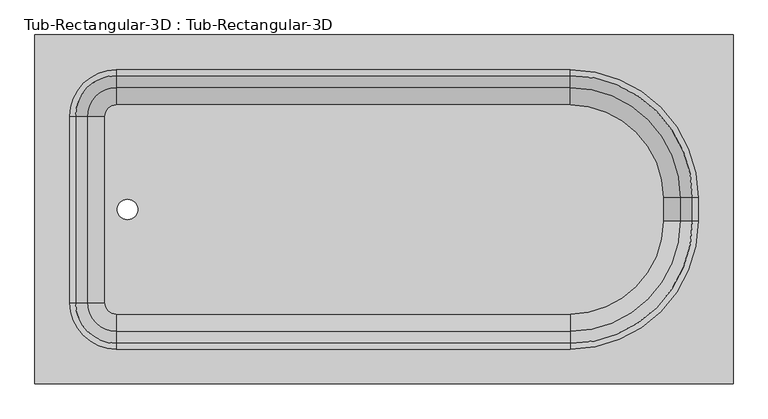
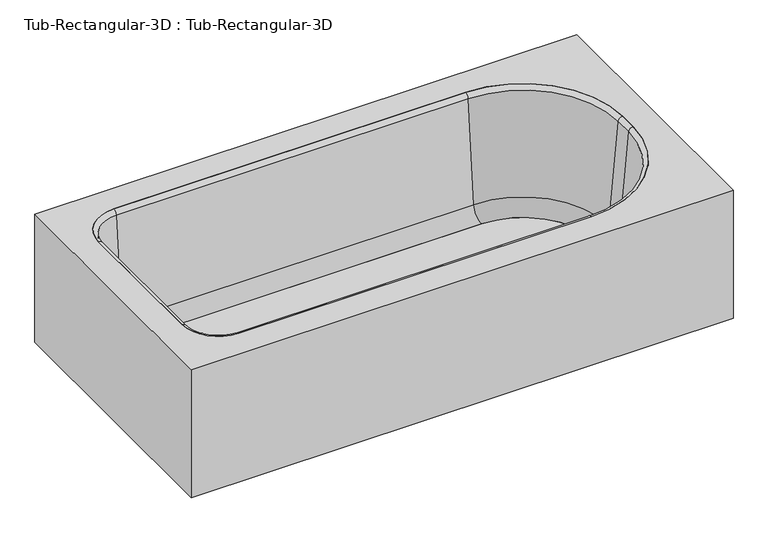
"""IFC4 building model written with IfcOpenShell, lengths in millimetres: flow terminal geometry, Tub-Rectangular-3D : Tub-Rectangular-3D."""

from ifc_helpers import new_model, si_unit, point, frame, frame_2d, origin, place, context, project, spatial, polyline, circle_curve, ellipse_curve, trimmed, segment, composite_curve, outline, extrude, source, transform, mapped, element, save
from ifc_brep_helpers import plane_surface, cylinder_surface, revolved_surface, advanced_brep


def tub_rectangular_3d_tub_rectangular_3d_36e24cee(model_context):
    return source(origin(), model_context, "Body", "SolidModel", [
        advanced_brep(
        [(413.3970313, 838.2, 381.0), (-1110.6029687, 838.2, 381.0), (-1110.6029687, 76.2, 381.0), (413.3970313, 76.2, 381.0), (-932.8029687, 762.0, 381.0), (57.7970313, 762.0, 381.0), (337.1970313, 482.6, 381.0), (337.1970313, 431.8, 381.0), (57.7970313, 152.4, 381.0), (-932.8029687, 152.4, 381.0), (-1034.4029687, 254.0, 381.0), (-1034.4029687, 660.4, 381.0), (394.3470313, 819.15, 361.95), (394.3470313, 95.25, 361.95), (-1091.5529687, 95.25, 361.95), (-1091.5529687, 819.15, 361.95), (-932.8029687, 762.0, 361.95), (-1034.4029687, 660.4, 361.95), (-1034.4029687, 254.0, 361.95), (-932.8029687, 152.4, 361.95), (57.7970313, 152.4, 361.95), (337.1970313, 431.8, 361.95), (337.1970313, 482.6, 361.95), (57.7970313, 762.0, 361.95), (413.3970313, 838.2, 0.0), (-1110.6029687, 838.2, 0.0), (-1110.6029687, 76.2, 0.0), (413.3970313, 76.2, 0.0), (394.3470313, 819.15, 0.0), (-1091.5529687, 819.15, 0.0), (-1091.5529687, 95.25, 0.0), (394.3470313, 95.25, 0.0)],
        [
            (0, 1),
            (1, 2),
            (2, 3),
            (3, 0),
            (4, 5),
            (5, 6, circle_curve(frame((57.7970313, 482.6, 381.0), z_axis=(0.0, 0.0, -1.0), x_axis=(0.0, 1.0, 0.0)), 279.4)),
            (6, 7),
            (7, 8, circle_curve(frame((57.7970313, 431.8, 381.0), z_axis=(0.0, 0.0, -1.0), x_axis=(0.0, 1.0, 0.0)), 279.4)),
            (8, 9),
            (9, 10, circle_curve(frame((-932.8029687, 254.0, 381.0), z_axis=(0.0, 0.0, -1.0), x_axis=(0.0, 1.0, 0.0)), 101.6)),
            (10, 11),
            (11, 4, circle_curve(frame((-932.8029687, 660.4, 381.0), z_axis=(0.0, 0.0, -1.0), x_axis=(0.0, 1.0, 0.0)), 101.6)),
            (12, 13),
            (13, 14),
            (14, 15),
            (15, 12),
            (16, 17, circle_curve(frame((-932.8029687, 660.4, 361.95), z_axis=(0.0, 0.0, 1.0), x_axis=(0.0, 1.0, 0.0)), 101.6)),
            (17, 18),
            (18, 19, circle_curve(frame((-932.8029687, 254.0, 361.95), z_axis=(0.0, 0.0, 1.0), x_axis=(0.0, 1.0, 0.0)), 101.6)),
            (19, 20),
            (20, 21, circle_curve(frame((57.7970313, 431.8, 361.95), z_axis=(0.0, 0.0, 1.0), x_axis=(0.0, 1.0, 0.0)), 279.4)),
            (21, 22),
            (22, 23, circle_curve(frame((57.7970313, 482.6, 361.95), z_axis=(0.0, 0.0, 1.0), x_axis=(0.0, 1.0, 0.0)), 279.4)),
            (23, 16),
            (0, 24),
            (24, 25),
            (25, 1),
            (25, 26),
            (26, 2),
            (26, 27),
            (27, 3),
            (27, 24),
            (4, 16),
            (23, 5),
            (22, 6),
            (21, 7),
            (20, 8),
            (19, 9),
            (18, 10),
            (17, 11),
            (28, 29),
            (29, 30),
            (30, 31),
            (31, 28),
            (31, 13),
            (12, 28),
            (30, 14),
            (29, 15),
        ],
        [
            plane_surface(frame((-1110.6029687, 838.2, 381.0), z_axis=(0.0, 0.0, 1.0), x_axis=(-1.0, 0.0, 0.0))),
            plane_surface(frame((-1110.6029687, 838.2, 361.95), z_axis=(0.0, 0.0, -1.0), x_axis=(1.0, 0.0, 0.0))),
            plane_surface(frame((413.3970313, 838.2, 381.0), z_axis=(0.0, 1.0, 0.0), x_axis=(0.0, 0.0, -1.0))),
            plane_surface(frame((-1110.6029687, 838.2, 381.0), z_axis=(-1.0, 0.0, 0.0), x_axis=(0.0, 0.0, -1.0))),
            plane_surface(frame((-1110.6029687, 76.2, 381.0), z_axis=(0.0, -1.0, 0.0), x_axis=(0.0, 0.0, -1.0))),
            plane_surface(frame((413.3970313, 76.2, 381.0), z_axis=(1.0, 0.0, 0.0), x_axis=(0.0, 0.0, -1.0))),
            plane_surface(frame((-932.8029687, 762.0, 381.0), z_axis=(0.0, -1.0, 0.0), x_axis=(0.0, 0.0, -1.0))),
            revolved_surface(polyline([(57.7970313, 762.0, 361.95), (57.7970313, 762.0, 381.0)]), (57.7970313, 482.6, 381.0), (0.0, 0.0, -1.0)),
            plane_surface(frame((337.1970313, 482.6, 381.0), z_axis=(-1.0, 0.0, 0.0), x_axis=(0.0, 0.0, -1.0))),
            revolved_surface(polyline([(57.7970313, 711.2, 361.95), (57.7970313, 711.2, 381.0)]), (57.7970313, 431.8, 381.0), (0.0, 0.0, -1.0)),
            plane_surface(frame((57.7970313, 152.4, 381.0), z_axis=(0.0, 1.0, 0.0), x_axis=(0.0, 0.0, -1.0))),
            revolved_surface(polyline([(-932.8029687, 355.6, 361.95), (-932.8029687, 355.6, 381.0)]), (-932.8029687, 254.0, 381.0), (0.0, 0.0, -1.0)),
            plane_surface(frame((-1034.4029687, 254.0, 381.0), z_axis=(1.0, 0.0, 0.0), x_axis=(0.0, 0.0, -1.0))),
            revolved_surface(polyline([(-932.8029687, 762.0, 361.95), (-932.8029687, 762.0, 381.0)]), (-932.8029687, 660.4, 381.0), (0.0, 0.0, -1.0)),
            plane_surface(frame((-1110.6029687, 838.2, 0.0), z_axis=(0.0, 0.0, -1.0), x_axis=(1.0, 0.0, 0.0))),
            plane_surface(frame((394.3470313, 819.15, 361.95), z_axis=(-1.0, 0.0, 0.0), x_axis=(0.0, 0.0, -1.0))),
            plane_surface(frame((394.3470313, 95.25, 361.95), z_axis=(0.0, 1.0, 0.0), x_axis=(0.0, 0.0, -1.0))),
            plane_surface(frame((-1091.5529687, 95.25, 361.95), z_axis=(1.0, 0.0, 0.0), x_axis=(0.0, 0.0, -1.0))),
            plane_surface(frame((-1091.5529687, 819.15, 361.95), z_axis=(0.0, -1.0, 0.0), x_axis=(0.0, 0.0, -1.0))),
        ],
        [
            (0, [[1, 2, 3, 4], [5, 6, 7, 8, 9, 10, 11, 12]]),
            (1, [[13, 14, 15, 16], [17, 18, 19, 20, 21, 22, 23, 24]]),
            (2, [[-1, 25, 26, 27]]),
            (3, [[-2, -27, 28, 29]]),
            (4, [[-3, -29, 30, 31]]),
            (5, [[-25, -4, -31, 32]]),
            (6, [[-5, 33, -24, 34]]),
            (7, [[-6, -34, -23, 35]]),
            (8, [[-7, -35, -22, 36]]),
            (9, [[-8, -36, -21, 37]]),
            (10, [[-9, -37, -20, 38]]),
            (11, [[-10, -38, -19, 39]]),
            (12, [[-11, -39, -18, 40]]),
            (13, [[-12, -40, -17, -33]]),
            (14, [[-32, -30, -28, -26], [41, 42, 43, 44]]),
            (15, [[-44, 45, -13, 46]]),
            (16, [[-43, 47, -14, -45]]),
            (17, [[-42, 48, -15, -47]]),
            (18, [[-41, -46, -16, -48]]),
        ],
    ),
        extrude(outline(composite_curve([segment(trimmed(circle_curve(frame_2d((57.7970313, 482.6)), 202.7964741), [point((57.7970313, 685.3964741))], [point((260.5935054, 482.6))], False, "CARTESIAN"), True, "CONTINUOUS"), segment(polyline([(260.5935054, 482.6), (260.5935054, 431.8)]), True, "CONTINUOUS"), segment(trimmed(circle_curve(frame_2d((57.7970313, 431.8)), 202.7964741), [point((260.5935054, 431.8))], [point((57.7970313, 229.0035259))], False, "CARTESIAN"), True, "CONTINUOUS"), segment(polyline([(57.7970313, 229.0035259), (-932.8029687, 229.0035259)]), True, "CONTINUOUS"), segment(trimmed(circle_curve(frame_2d((-932.8029687, 254.0)), 24.9964741), [point((-932.8029687, 229.0035259))], [point((-957.7994428, 254.0))], False, "CARTESIAN"), True, "CONTINUOUS"), segment(polyline([(-957.7994428, 254.0), (-957.7994428, 660.4)]), True, "CONTINUOUS"), segment(trimmed(circle_curve(frame_2d((-932.8029687, 660.4)), 24.9964741), [point((-957.7994428, 660.4))], [point((-932.8029687, 685.3964741))], False, "CARTESIAN"), True, "CONTINUOUS"), segment(polyline([(-932.8029687, 685.3964741), (57.7970313, 685.3964741)]), True, "CONTINUOUS")], self_intersect=False), holes=[composite_curve([segment(trimmed(circle_curve(frame_2d((-908.510206, 457.2)), 22.225), [point((-908.510206, 479.425))], [point((-908.510206, 434.975))], True, "CARTESIAN"), True, "CONTINUOUS"), segment(trimmed(circle_curve(frame_2d((-908.510206, 457.2)), 22.225), [point((-908.510206, 434.975))], [point((-908.510206, 479.425))], True, "CARTESIAN"), True, "CONTINUOUS")], self_intersect=False)]), frame((0.0, 0.0, 16.863573), z_axis=(0.0, 0.0, 1.0), x_axis=(1.0, 0.0, 0.0)), (0.0, 0.0, 1.0), 19.05),
        advanced_brep(
        [(-995.7544608, 660.4, 70.6929392), (-932.8029687, 723.3514921, 70.6929392), (-932.8029687, 749.5220035, 369.8232535), (-1021.9249722, 660.4, 369.8232535), (-957.7994428, 660.4, 35.913573), (-932.8029687, 685.3964741, 35.913573), (-957.7994428, 660.4, 16.863573), (-932.8029687, 685.3964741, 16.863573), (-1034.4029687, 660.4, 16.863573), (-932.8029687, 762.0, 16.863573), (-1034.4029687, 660.4, 381.0), (-932.8029687, 762.0, 381.0), (-1021.9249722, 254.0, 369.8232535), (-995.7544608, 254.0, 70.6929392), (-957.7994428, 254.0, 35.913573), (-957.7994428, 254.0, 16.863573), (-1034.4029687, 254.0, 16.863573), (-1034.4029687, 254.0, 381.0), (-932.8029687, 191.0485079, 70.6929392), (-932.8029687, 164.8779965, 369.8232535), (-932.8029687, 229.0035259, 35.913573), (-932.8029687, 229.0035259, 16.863573), (-932.8029687, 152.4, 16.863573), (-932.8029687, 152.4, 381.0), (57.7970313, 164.8779965, 369.8232535), (57.7970313, 191.0485079, 70.6929392), (57.7970313, 229.0035259, 35.913573), (57.7970313, 229.0035259, 16.863573), (57.7970313, 152.4, 16.863573), (57.7970313, 152.4, 381.0), (298.5485234, 431.8, 70.6929392), (324.7190348, 431.8, 369.8232535), (260.5935054, 431.8, 35.913573), (260.5935054, 431.8, 16.863573), (337.1970313, 431.8, 16.863573), (337.1970313, 431.8, 381.0), (324.7190348, 482.6, 369.8232535), (298.5485234, 482.6, 70.6929392), (260.5935054, 482.6, 35.913573), (260.5935054, 482.6, 16.863573), (337.1970313, 482.6, 16.863573), (337.1970313, 482.6, 381.0), (57.7970313, 723.3514921, 70.6929392), (57.7970313, 749.5220035, 369.8232535), (57.7970313, 685.3964741, 35.913573), (57.7970313, 685.3964741, 16.863573), (57.7970313, 762.0, 16.863573), (57.7970313, 762.0, 381.0)],
        [
            (0, 1, circle_curve(frame((-932.8029687, 660.4, 70.6929392), z_axis=(0.0, 0.0, -1.0), x_axis=(0.0, 1.0, 0.0)), 62.9514921)),
            (1, 2),
            (2, 3, circle_curve(frame((-932.8029687, 660.4, 369.8232535), z_axis=(0.0, 0.0, 1.0), x_axis=(0.0, 1.0, 0.0)), 89.1220035)),
            (3, 0),
            (4, 5, circle_curve(frame((-932.8029687, 660.4, 35.913573), z_axis=(0.0, 0.0, -1.0), x_axis=(0.0, 1.0, 0.0)), 24.9964741)),
            (5, 1, circle_curve(frame((-932.8029687, 685.3964741, 74.013573), z_axis=(1.0, 0.0, 0.0), x_axis=(0.0, -1.0, 0.0)), 38.1)),
            (0, 4, circle_curve(frame((-957.7994428, 660.4, 74.013573), z_axis=(0.0, -1.0, 0.0), x_axis=(1.0, 0.0, 0.0)), 38.1)),
            (6, 7, circle_curve(frame((-932.8029687, 660.4, 16.863573), z_axis=(0.0, 0.0, -1.0), x_axis=(0.0, 1.0, 0.0)), 24.9964741)),
            (7, 5),
            (4, 6),
            (8, 9, circle_curve(frame((-932.8029687, 660.4, 16.863573), z_axis=(0.0, 0.0, -1.0), x_axis=(0.0, 1.0, 0.0)), 101.6)),
            (9, 7),
            (6, 8),
            (10, 11, circle_curve(frame((-932.8029687, 660.4, 381.0), z_axis=(0.0, 0.0, -1.0), x_axis=(0.0, 1.0, 0.0)), 101.6)),
            (11, 9),
            (8, 10),
            (2, 11, circle_curve(frame((-932.8029687, 762.0, 368.4462547), z_axis=(-1.0, 0.0, 0.0), x_axis=(0.0, -1.0, 0.0)), 12.5537453)),
            (10, 3, circle_curve(frame((-1034.4029687, 660.4, 368.4462547), z_axis=(0.0, 1.0, 0.0), x_axis=(1.0, 0.0, 0.0)), 12.5537453)),
            (3, 12),
            (12, 13),
            (13, 0),
            (13, 14, circle_curve(frame((-957.7994428, 254.0, 74.013573), z_axis=(0.0, -1.0, 0.0), x_axis=(1.0, 0.0, 0.0)), 38.1)),
            (14, 4),
            (14, 15),
            (15, 6),
            (15, 16),
            (16, 8),
            (16, 17),
            (17, 10),
            (17, 12, circle_curve(frame((-1034.4029687, 254.0, 368.4462547), z_axis=(0.0, 1.0, 0.0), x_axis=(1.0, 0.0, 0.0)), 12.5537453)),
            (18, 13, circle_curve(frame((-932.8029687, 254.0, 70.6929392), z_axis=(0.0, 0.0, -1.0), x_axis=(-1.0, 0.0, 0.0)), 62.9514921)),
            (12, 19, circle_curve(frame((-932.8029687, 254.0, 369.8232535), z_axis=(0.0, 0.0, 1.0), x_axis=(-1.0, 0.0, 0.0)), 89.1220035)),
            (19, 18),
            (20, 14, circle_curve(frame((-932.8029687, 254.0, 35.913573), z_axis=(0.0, 0.0, -1.0), x_axis=(-1.0, 0.0, 0.0)), 24.9964741)),
            (18, 20, circle_curve(frame((-932.8029687, 229.0035259, 74.013573), z_axis=(1.0, 0.0, 0.0), x_axis=(0.0, 1.0, 0.0)), 38.1)),
            (21, 15, circle_curve(frame((-932.8029687, 254.0, 16.863573), z_axis=(0.0, 0.0, -1.0), x_axis=(-1.0, 0.0, 0.0)), 24.9964741)),
            (20, 21),
            (22, 16, circle_curve(frame((-932.8029687, 254.0, 16.863573), z_axis=(0.0, 0.0, -1.0), x_axis=(-1.0, 0.0, 0.0)), 101.6)),
            (21, 22),
            (23, 17, circle_curve(frame((-932.8029687, 254.0, 381.0), z_axis=(0.0, 0.0, -1.0), x_axis=(-1.0, 0.0, 0.0)), 101.6)),
            (22, 23),
            (23, 19, circle_curve(frame((-932.8029687, 152.4, 368.4462547), z_axis=(-1.0, 0.0, 0.0), x_axis=(0.0, 1.0, 0.0)), 12.5537453)),
            (19, 24),
            (24, 25),
            (25, 18),
            (25, 26, circle_curve(frame((57.7970313, 229.0035259, 74.013573), z_axis=(1.0, 0.0, 0.0), x_axis=(0.0, 1.0, 0.0)), 38.1)),
            (26, 20),
            (26, 27),
            (27, 21),
            (27, 28),
            (28, 22),
            (28, 29),
            (29, 23),
            (29, 24, circle_curve(frame((57.7970313, 152.4, 368.4462547), z_axis=(-1.0, 0.0, 0.0), x_axis=(0.0, 1.0, 0.0)), 12.5537453)),
            (30, 25, circle_curve(frame((57.7970313, 431.8, 70.6929392), z_axis=(0.0, 0.0, -1.0), x_axis=(0.0, -1.0, 0.0)), 240.7514921)),
            (24, 31, circle_curve(frame((57.7970313, 431.8, 369.8232535), z_axis=(0.0, 0.0, 1.0), x_axis=(0.0, -1.0, 0.0)), 266.9220035)),
            (31, 30),
            (32, 26, circle_curve(frame((57.7970313, 431.8, 35.913573), z_axis=(0.0, 0.0, -1.0), x_axis=(0.0, -1.0, 0.0)), 202.7964741)),
            (30, 32, circle_curve(frame((260.5935054, 431.8, 74.013573), z_axis=(0.0, 1.0, 0.0), x_axis=(-1.0, 0.0, 0.0)), 38.1)),
            (33, 27, circle_curve(frame((57.7970313, 431.8, 16.863573), z_axis=(0.0, 0.0, -1.0), x_axis=(0.0, -1.0, 0.0)), 202.7964741)),
            (32, 33),
            (34, 28, circle_curve(frame((57.7970313, 431.8, 16.863573), z_axis=(0.0, 0.0, -1.0), x_axis=(0.0, -1.0, 0.0)), 279.4)),
            (33, 34),
            (35, 29, circle_curve(frame((57.7970313, 431.8, 381.0), z_axis=(0.0, 0.0, -1.0), x_axis=(0.0, -1.0, 0.0)), 279.4)),
            (34, 35),
            (35, 31, circle_curve(frame((337.1970313, 431.8, 368.4462547), z_axis=(0.0, -1.0, 0.0), x_axis=(-1.0, 0.0, 0.0)), 12.5537453)),
            (31, 36),
            (36, 37),
            (37, 30),
            (37, 38, circle_curve(frame((260.5935054, 482.6, 74.013573), z_axis=(0.0, 1.0, 0.0), x_axis=(-1.0, 0.0, 0.0)), 38.1)),
            (38, 32),
            (38, 39),
            (39, 33),
            (39, 40),
            (40, 34),
            (40, 41),
            (41, 35),
            (41, 36, circle_curve(frame((337.1970313, 482.6, 368.4462547), z_axis=(0.0, -1.0, 0.0), x_axis=(-1.0, 0.0, 0.0)), 12.5537453)),
            (42, 37, circle_curve(frame((57.7970313, 482.6, 70.6929392), z_axis=(0.0, 0.0, -1.0), x_axis=(1.0, 0.0, 0.0)), 240.7514921)),
            (36, 43, circle_curve(frame((57.7970313, 482.6, 369.8232535), z_axis=(0.0, 0.0, 1.0), x_axis=(1.0, 0.0, 0.0)), 266.9220035)),
            (43, 42),
            (44, 38, circle_curve(frame((57.7970313, 482.6, 35.913573), z_axis=(0.0, 0.0, -1.0), x_axis=(1.0, 0.0, 0.0)), 202.7964741)),
            (42, 44, circle_curve(frame((57.7970313, 685.3964741, 74.013573), z_axis=(-1.0, 0.0, 0.0), x_axis=(0.0, -1.0, 0.0)), 38.1)),
            (45, 39, circle_curve(frame((57.7970313, 482.6, 16.863573), z_axis=(0.0, 0.0, -1.0), x_axis=(1.0, 0.0, 0.0)), 202.7964741)),
            (44, 45),
            (46, 40, circle_curve(frame((57.7970313, 482.6, 16.863573), z_axis=(0.0, 0.0, -1.0), x_axis=(1.0, 0.0, 0.0)), 279.4)),
            (45, 46),
            (47, 41, circle_curve(frame((57.7970313, 482.6, 381.0), z_axis=(0.0, 0.0, -1.0), x_axis=(1.0, 0.0, 0.0)), 279.4)),
            (46, 47),
            (47, 43, circle_curve(frame((57.7970313, 762.0, 368.4462547), z_axis=(1.0, 0.0, 0.0), x_axis=(0.0, -1.0, 0.0)), 12.5537453)),
            (43, 2),
            (1, 42),
            (5, 44),
            (7, 45),
            (9, 46),
            (11, 47),
        ],
        [
            revolved_surface(polyline([(-932.8029687, 749.5220035, 369.8232535), (-932.8029687, 723.3514921, 70.6929392)]), (-932.8029687, 660.4, 381.0), (0.0, 0.0, 1.0)),
            revolved_surface(trimmed(ellipse_curve(frame((-932.8029687, 685.3964741, 74.013573), z_axis=(-1.0, 0.0, 0.0), x_axis=(0.0, -1.0, 0.0)), 38.1, 38.1), [point((-932.8029687, 723.3514921, 70.6929392))], [point((-932.8029687, 685.3964741, 35.913573))], True, "CARTESIAN"), (-932.8029687, 660.4, 381.0), (0.0, 0.0, 1.0)),
            revolved_surface(polyline([(-932.8029687, 685.3964741, 35.913572999999985), (-932.8029687, 685.3964741, 16.863572999999974)]), (-932.8029687, 660.4, 381.0), (0.0, 0.0, 1.0)),
            plane_surface(frame((-932.8029687, 660.4, 16.863573), z_axis=(0.0, 0.0, -1.0), x_axis=(0.0, 1.0, 0.0))),
            cylinder_surface(frame((-932.8029687, 660.4, 381.0), z_axis=(0.0, 0.0, 1.0), x_axis=(0.0, 1.0, 0.0)), 101.6),
            revolved_surface(trimmed(ellipse_curve(frame((-932.8029687, 762.0, 368.4462547), z_axis=(1.0, 0.0, 0.0), x_axis=(0.0, -1.0, 0.0)), 12.5537453, 12.5537453), [point((-932.8029687, 762.0, 381.0))], [point((-932.8029687, 749.5220035, 369.8232535))], True, "CARTESIAN"), (-932.8029687, 660.4, 381.0), (0.0, 0.0, 1.0)),
            plane_surface(frame((-1021.9249722, 660.4, 369.8232535), z_axis=(0.9961946980917458, 0.0, 0.08715574274765626), x_axis=(0.0, -1.0, 0.0))),
            revolved_surface(polyline([(-919.6994427999999, 254.0, 74.013573), (-919.6994427999999, 660.4, 74.013573)]), (-957.7994428, 660.4, 74.013573), (0.0, -1.0, 0.0)),
            plane_surface(frame((-957.7994428, 660.4, 35.913573), z_axis=(1.0, 0.0, 0.0), x_axis=(0.0, -1.0, 0.0))),
            plane_surface(frame((-957.7994428, 660.4, 16.863573), z_axis=(0.0, 0.0, -1.0), x_axis=(0.0, -1.0, 0.0))),
            plane_surface(frame((-1034.4029687, 660.4, 16.863573), z_axis=(-1.0, 0.0, 0.0), x_axis=(0.0, -1.0, 0.0))),
            cylinder_surface(frame((-1034.4029687, 660.4, 368.4462547), z_axis=(0.0, 1.0, 0.0), x_axis=(1.0, 0.0, 0.0)), 12.5537453),
            revolved_surface(polyline([(-1021.9249722, 254.0, 369.8232535), (-995.7544608, 254.0, 70.6929392)]), (-932.8029687, 254.0, 381.0), (0.0, 0.0, 1.0)),
            revolved_surface(trimmed(ellipse_curve(frame((-957.7994428, 254.0, 74.013573), z_axis=(0.0, -1.0, 0.0), x_axis=(1.0, 0.0, 0.0)), 38.1, 38.1), [point((-995.7544608, 254.0, 70.6929392))], [point((-957.7994428, 254.0, 35.913573))], True, "CARTESIAN"), (-932.8029687, 254.0, 381.0), (0.0, 0.0, 1.0)),
            revolved_surface(polyline([(-957.7994428, 254.0, 35.913572999999985), (-957.7994428, 254.0, 16.863572999999974)]), (-932.8029687, 254.0, 381.0), (0.0, 0.0, 1.0)),
            plane_surface(frame((-932.8029687, 254.0, 16.863573), z_axis=(0.0, 0.0, -1.0), x_axis=(-1.0, 0.0, 0.0))),
            cylinder_surface(frame((-932.8029687, 254.0, 381.0), z_axis=(0.0, 0.0, 1.0), x_axis=(-1.0, 0.0, 0.0)), 101.6),
            revolved_surface(trimmed(ellipse_curve(frame((-1034.4029687, 254.0, 368.4462547), z_axis=(0.0, 1.0, 0.0), x_axis=(1.0, 0.0, 0.0)), 12.5537453, 12.5537453), [point((-1034.4029687, 254.0, 381.0))], [point((-1021.9249722, 254.0, 369.8232535))], True, "CARTESIAN"), (-932.8029687, 254.0, 381.0), (0.0, 0.0, 1.0)),
            plane_surface(frame((-932.8029687, 164.8779965, 369.8232535), z_axis=(0.0, 0.9961946980917461, 0.08715574274765303), x_axis=(1.0, 0.0, 0.0))),
            revolved_surface(polyline([(57.79703129999996, 267.1035259, 74.013573), (-932.8029687, 267.1035259, 74.013573)]), (-932.8029687, 229.0035259, 74.013573), (1.0, 0.0, 0.0)),
            plane_surface(frame((-932.8029687, 229.0035259, 35.913573), z_axis=(0.0, 1.0, 0.0), x_axis=(1.0, 0.0, 0.0))),
            plane_surface(frame((-932.8029687, 229.0035259, 16.863573), z_axis=(0.0, 0.0, -1.0), x_axis=(1.0, 0.0, 0.0))),
            plane_surface(frame((-932.8029687, 152.4, 16.863573), z_axis=(0.0, -1.0, 0.0), x_axis=(1.0, 0.0, 0.0))),
            cylinder_surface(frame((-932.8029687, 152.4, 368.4462547), z_axis=(-1.0, 0.0, 0.0), x_axis=(0.0, 1.0, 0.0)), 12.5537453),
            revolved_surface(polyline([(57.7970313, 164.8779965, 369.8232535), (57.7970313, 191.0485079, 70.6929392)]), (57.7970313, 431.8, 381.0), (0.0, 0.0, 1.0)),
            revolved_surface(trimmed(ellipse_curve(frame((57.7970313, 229.0035259, 74.013573), z_axis=(1.0, 0.0, 0.0), x_axis=(0.0, 1.0, 0.0)), 38.1, 38.1), [point((57.7970313, 191.0485079, 70.6929392))], [point((57.7970313, 229.0035259, 35.913573))], True, "CARTESIAN"), (57.7970313, 431.8, 381.0), (0.0, 0.0, 1.0)),
            revolved_surface(polyline([(57.7970313, 229.0035259, 35.913572999999985), (57.7970313, 229.0035259, 16.863572999999974)]), (57.7970313, 431.8, 381.0), (0.0, 0.0, 1.0)),
            plane_surface(frame((57.7970313, 431.8, 16.863573), z_axis=(0.0, 0.0, -1.0), x_axis=(0.0, -1.0, 0.0))),
            cylinder_surface(frame((57.7970313, 431.8, 381.0), z_axis=(0.0, 0.0, 1.0), x_axis=(0.0, -1.0, 0.0)), 279.4),
            revolved_surface(trimmed(ellipse_curve(frame((57.7970313, 152.4, 368.4462547), z_axis=(-1.0, 0.0, 0.0), x_axis=(0.0, 1.0, 0.0)), 12.5537453, 12.5537453), [point((57.7970313, 152.4, 381.0))], [point((57.7970313, 164.8779965, 369.8232535))], True, "CARTESIAN"), (57.7970313, 431.8, 381.0), (0.0, 0.0, 1.0)),
            plane_surface(frame((324.7190348, 431.8, 369.8232535), z_axis=(-0.9961946980917463, 0.0, 0.0871557427476498), x_axis=(0.0, 1.0, 0.0))),
            revolved_surface(polyline([(222.49350540000003, 482.6, 74.013573), (222.49350540000003, 431.8, 74.013573)]), (260.5935054, 431.8, 74.013573), (0.0, 1.0, 0.0)),
            plane_surface(frame((260.5935054, 431.8, 35.913573), z_axis=(-1.0, 0.0, 0.0), x_axis=(0.0, 1.0, 0.0))),
            plane_surface(frame((260.5935054, 431.8, 16.863573), z_axis=(0.0, 0.0, -1.0), x_axis=(0.0, 1.0, 0.0))),
            plane_surface(frame((337.1970313, 431.8, 16.863573), z_axis=(1.0, 0.0, 0.0), x_axis=(0.0, 1.0, 0.0))),
            cylinder_surface(frame((337.1970313, 431.8, 368.4462547), z_axis=(0.0, -1.0, 0.0), x_axis=(-1.0, 0.0, 0.0)), 12.5537453),
            revolved_surface(polyline([(324.7190348, 482.6, 369.8232535), (298.5485234, 482.6, 70.6929392)]), (57.7970313, 482.6, 381.0), (0.0, 0.0, 1.0)),
            revolved_surface(trimmed(ellipse_curve(frame((260.5935054, 482.6, 74.013573), z_axis=(0.0, 1.0, 0.0), x_axis=(-1.0, 0.0, 0.0)), 38.1, 38.1), [point((298.5485234, 482.6, 70.6929392))], [point((260.5935054, 482.6, 35.913573))], True, "CARTESIAN"), (57.7970313, 482.6, 381.0), (0.0, 0.0, 1.0)),
            revolved_surface(polyline([(260.5935054, 482.6, 35.913572999999985), (260.5935054, 482.6, 16.863572999999974)]), (57.7970313, 482.6, 381.0), (0.0, 0.0, 1.0)),
            plane_surface(frame((57.7970313, 482.6, 16.863573), z_axis=(0.0, 0.0, -1.0), x_axis=(1.0, 0.0, 0.0))),
            cylinder_surface(frame((57.7970313, 482.6, 381.0), z_axis=(0.0, 0.0, 1.0), x_axis=(1.0, 0.0, 0.0)), 279.4),
            revolved_surface(trimmed(ellipse_curve(frame((337.1970313, 482.6, 368.4462547), z_axis=(0.0, -1.0, 0.0), x_axis=(-1.0, 0.0, 0.0)), 12.5537453, 12.5537453), [point((337.1970313, 482.6, 381.0))], [point((324.7190348, 482.6, 369.8232535))], True, "CARTESIAN"), (57.7970313, 482.6, 381.0), (0.0, 0.0, 1.0)),
            plane_surface(frame((57.7970313, 749.5220035, 369.8232535), z_axis=(0.0, -0.996194698091746, 0.08715574274765303), x_axis=(-1.0, 0.0, 0.0))),
            revolved_surface(polyline([(-932.8029687, 647.2964741, 74.013573), (57.7970313, 647.2964741, 74.013573)]), (57.7970313, 685.3964741, 74.013573), (-1.0, 0.0, 0.0)),
            plane_surface(frame((57.7970313, 685.3964741, 35.913573), z_axis=(0.0, -1.0, 0.0), x_axis=(-1.0, 0.0, 0.0))),
            plane_surface(frame((57.7970313, 685.3964741, 16.863573), z_axis=(0.0, 0.0, -1.0), x_axis=(-1.0, 0.0, 0.0))),
            plane_surface(frame((57.7970313, 762.0, 16.863573), z_axis=(0.0, 1.0, 0.0), x_axis=(-1.0, 0.0, 0.0))),
            cylinder_surface(frame((57.7970313, 762.0, 368.4462547), z_axis=(1.0, 0.0, 0.0), x_axis=(0.0, -1.0, 0.0)), 12.5537453),
        ],
        [
            (0, [[1, 2, 3, 4]]),
            (1, [[5, 6, -1, 7]]),
            (2, [[8, 9, -5, 10]]),
            (3, [[11, 12, -8, 13]]),
            (4, [[14, 15, -11, 16]]),
            (5, [[-3, 17, -14, 18]]),
            (6, [[-4, 19, 20, 21]]),
            (7, [[-7, -21, 22, 23]]),
            (8, [[-10, -23, 24, 25]]),
            (9, [[-13, -25, 26, 27]]),
            (10, [[-16, -27, 28, 29]]),
            (11, [[-18, -29, 30, -19]]),
            (12, [[31, -20, 32, 33]]),
            (13, [[34, -22, -31, 35]]),
            (14, [[36, -24, -34, 37]]),
            (15, [[38, -26, -36, 39]]),
            (16, [[40, -28, -38, 41]]),
            (17, [[-32, -30, -40, 42]]),
            (18, [[-33, 43, 44, 45]]),
            (19, [[-35, -45, 46, 47]]),
            (20, [[-37, -47, 48, 49]]),
            (21, [[-39, -49, 50, 51]]),
            (22, [[-41, -51, 52, 53]]),
            (23, [[-42, -53, 54, -43]]),
            (24, [[55, -44, 56, 57]]),
            (25, [[58, -46, -55, 59]]),
            (26, [[60, -48, -58, 61]]),
            (27, [[62, -50, -60, 63]]),
            (28, [[64, -52, -62, 65]]),
            (29, [[-56, -54, -64, 66]]),
            (30, [[-57, 67, 68, 69]]),
            (31, [[-59, -69, 70, 71]]),
            (32, [[-61, -71, 72, 73]]),
            (33, [[-63, -73, 74, 75]]),
            (34, [[-65, -75, 76, 77]]),
            (35, [[-66, -77, 78, -67]]),
            (36, [[79, -68, 80, 81]]),
            (37, [[82, -70, -79, 83]]),
            (38, [[84, -72, -82, 85]]),
            (39, [[86, -74, -84, 87]]),
            (40, [[88, -76, -86, 89]]),
            (41, [[-80, -78, -88, 90]]),
            (42, [[-81, 91, -2, 92]]),
            (43, [[-83, -92, -6, 93]]),
            (44, [[-85, -93, -9, 94]]),
            (45, [[-87, -94, -12, 95]]),
            (46, [[-89, -95, -15, 96]]),
            (47, [[-90, -96, -17, -91]]),
        ],
    ),
    ])


if __name__ == "__main__":
    model = new_model("IFC4")
    model_context = context("Model", 3, world=origin())
    ifc_project = project(units=[si_unit("LENGTHUNIT", "METRE", prefix="MILLI")], contexts=[model_context])
    site = spatial("IfcSite", under=ifc_project)
    building = spatial("IfcBuilding", under=site)
    placement = place(None, origin())
    tub_rectangular_3d_tub_rectangular_3d_shape = tub_rectangular_3d_tub_rectangular_3d_36e24cee(model_context)
    element("IfcFlowTerminal", 1, ObjectType="Tub-Rectangular-3D : Tub-Rectangular-3D", at=placement, inside=building, context=model_context, shape_type="MappedRepresentation", body=[
        mapped(tub_rectangular_3d_tub_rectangular_3d_shape, transform((0.0, 0.0, 0.0), x_axis=(1.0, 0.0, 0.0), y_axis=(0.0, 1.0, 0.0), z_axis=(0.0, 0.0, 1.0))),
    ])
    save(model, "model.ifc")

# Revit data of these elements
# Type "Tub-Rectangular-3D : Tub-Rectangular-3D"
#   Assembly Code = "D2010500"
#   Depth = 2' - 6"
#   Height = 1' - 3"
#   Width = 5' - 0"
#   Tub Material = Porcelain, Ivory
#   Default Elevation = 0
# Element 1 (IfcFlowTerminal, "Tub-Rectangular-3D : Tub-Rectangular-3D")
#   Materials on its faces: "Porcelain, Ivory"
# Materials
#   "Porcelain, Ivory": class "Ceramic", colour RGB 247 247 239, transparency 0, Description = "Porcelain, ivory", Cost = 0
